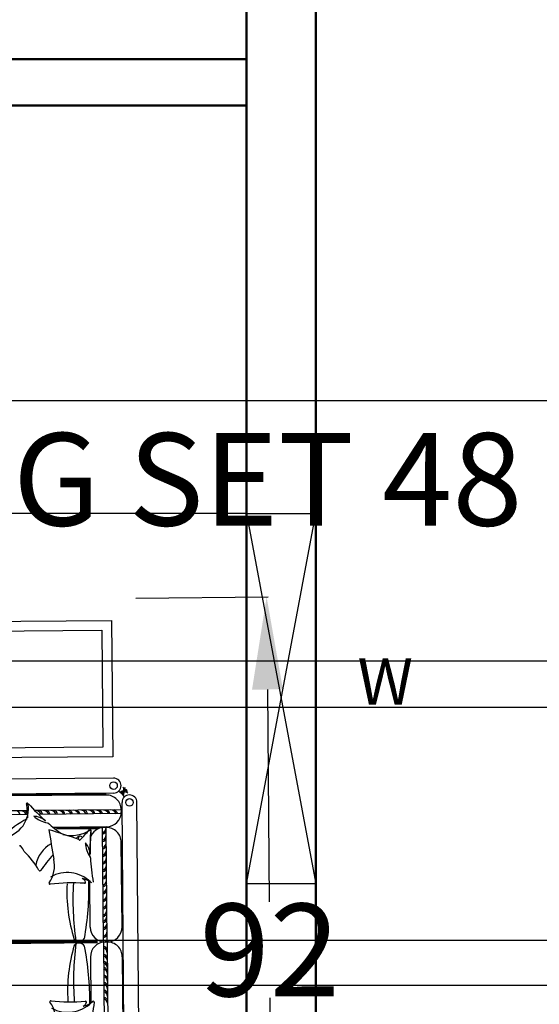
# Model space of a CAD drawing. Units: inches. Extents: x -77 to 516, y -119 to 536.
# Tile 9 of 11: x 335 to 403, y 159 to 287. Entities that reach past the tile are written whole.
import ezdxf

# ---------------------------------------------------------------- set-up
doc = ezdxf.new("R2010")
doc.units = ezdxf.units.IN
doc.header["$MEASUREMENT"] = 0
for name, color, linetype, lineweight in [('A-ANNO-DIMS', 2, 'Continuous', 18), ('furniture', 119, 'Continuous', 18), ('text', 170, 'Continuous', 18), ('walls', 40, 'Continuous', 50), ('windows', 1, 'Continuous', 25)]:
    doc.layers.add(name, color=color, linetype=linetype, lineweight=lineweight)
doc.layers.add('FUR', color=42, linetype='Continuous')
doc.styles.get("Standard").update_dxf_attribs({"font": 'arial.ttf'})
doc.dimstyles.get("Standard").update_dxf_attribs({"dimtxt": 12, "dimasz": 12, "dimexe": 0.18, "dimexo": 0.0625, "dimgap": 0.09, "dimtad": 0, "dimtih": 1, "dimtoh": 1, "dimdec": 1, "dimzin": 0, "dimdsep": 46, "dimlunit": 4, "dimtxsty": 'Standard', "dimcen": 0.09, "dimadec": 0, "dimazin": 0, "dimtfac": 1, "dimtdec": 1, "dimtofl": 0, "dimtmove": 0, "dimatfit": 3, "dimfxl": 1, "dimtolj": 1, "dimtzin": 0, "dimarcsym": 0})

# ---------------------------------------------------------------- blocks, each defined once
blk = doc.blocks.new('A$C44A37715')
at = {"layer": 'FUR'}
for p, q in [((0, 2.4786), (0, 1.048)), ((0.0768, 2.4786), (0.0768, 1.048)), ((0.1591, 1.763), (0.1591, 2.3508)), ((0.1783, 1.7636), (0.1783, 2.3502)), ((0.0822, 1.8399), (0.0822, 2.274)), ((0.2455, 1.8399), (0.2455, 2.0753)), ((0.1591, 1.764), (0.1687, 1.764)), ((0.1591, 1.764), (0.1687, 1.764)), ((0.1591, 1.7636), (0.1687, 1.7636)), ((0.1591, 1.7636), (0.1687, 1.7636)), ((0.1591, 1.7636), (0.1591, 1.1758)), ((0.1591, 1.763), (0.1687, 1.763)), ((0.1591, 1.7623), (0.1687, 1.7623)), ((0.1591, 1.7623), (0.1687, 1.7623)), ((0.1783, 1.763), (0.1783, 1.1764)), ((0.2091, 1.7681), (0.8452, 1.7681)), ((0.2091, 1.7681), (0.8452, 1.7681)), ((0.2091, 1.7633), (0.8487, 1.7633)), ((0.2091, 1.7585), (0.8452, 1.7585)), ((0.2103, 1.7681), (0.8452, 1.7681)), ((0.0822, 1.6868), (0.0822, 1.2527)), ((0.2455, 1.6868), (0.2455, 1.4514)), ((0.2446, 1.3239), (0.2446, 1.2958)), ((0.1577, 1.1727), (0.4308, 1.1727)), ((0.1591, 1.1758), (0.1687, 1.1758)), ((0.1845, 1.1775), (0.4249, 1.1775)), ((0.1995, 1.1823), (0.4138, 1.1823)), ((0.0809, 1.0862), (0.0809, 1.0958)), ((0.0809, 1.0862), (0.524, 1.0862)), ((0.0815, 1.1054), (0.5053, 1.1054)), ((0.5573, 1.0862), (0.8644, 1.0862)), ((0.56, 1.1054), (0.8638, 1.1054)), ((0.0809, 0.9614), (0.0809, 0.9614)), ((0.1193, 0.9998), (0.8259, 0.9998)), ((0.1577, 1.0094), (0.7875, 1.0094)), ((0.1577, 1.0046), (0.7875, 1.0046)), ((0.1193, 0.923), (0.8259, 0.923)), ((0.1193, 0.923), (0.8259, 0.923))]:
    blk.add_line(p, q, dxfattribs=at)
for points in [[(0.1226, 0.1134), (0.1226, 0.8134), (0.8226, 0.8134), (0.8226, 0.1134)], [(0.1726, 0.1634), (0.1726, 0.7634), (0.7726, 0.7634), (0.7726, 0.1634)]]:
    blk.add_lwpolyline(points, close=True, dxfattribs=at)
for centre in [(0.0384, 1.048), (0.1193, 0.9614)]:
    blk.add_circle(centre, 0.0192, dxfattribs=at)
for centre, radius, start, end in [((-0.7557, 2.2433), 0.9988, 350.147, 357.3879), ((0.5796, 2.1587), 0.1531, 167.3915, 215.6783), ((0.3624, 1.9521), 0.1703, 60.2042, 134.6584), ((0.1884, 2.0828), 0.0293, 181.8064, 249.8645), ((0.2331, 2.0716), 0.0048, 170.147, 311.7497), ((0.3028, 1.9936), 0.0998, 100.2155, 131.7497), ((1.732, 2.053), 1.4814, 179.0056, 190.4975), ((0.2725, 2.0713), 0.0048, 161.7015, 277.2637), ((0.2981, 2.0629), 0.0317, 114.2109, 161.7015), ((0.1823, 2.0725), 0.0245, 198.4382, 260.6098), ((0.1884, 2.0444), 0.0293, 181.8064, 249.8645), ((0.1823, 2.0341), 0.0245, 198.4382, 260.6098), ((0.3436, 1.1012), 0.9679, 83.706, 94.1744), ((-1.1315, 1.9749), 1.465, 351.9647, 3.6704), ((-0.4253, 2.0161), 0.7895, 342.552, 3.574), ((0.4506, 2.068), 0.0048, 259.041, 17.2752), ((0.1884, 2.006), 0.0293, 181.8064, 249.8645), ((0.1823, 1.9956), 0.0245, 198.4382, 260.6098), ((0.1884, 1.9676), 0.0293, 181.8064, 249.8645), ((0.1823, 1.9572), 0.0245, 198.4382, 260.6098), ((0.1884, 1.9292), 0.0293, 181.8064, 249.8645), ((0.1823, 1.9188), 0.0245, 198.4382, 260.6098), ((0.1884, 1.8972), 0.0293, 181.8064, 249.8645), ((0.1823, 1.8869), 0.0245, 198.4382, 260.6098), ((0.1591, 1.8399), 0.0768, 180, 270), ((0.1884, 1.8614), 0.0293, 181.8064, 249.8645), ((0.1823, 1.851), 0.0245, 198.4382, 260.6098), ((0.1884, 1.8204), 0.0293, 181.8064, 249.8645), ((0.1687, 1.8399), 0.0768, 270, 0), ((0.1823, 1.81), 0.0245, 198.4382, 260.6098), ((0.3031, 1.8009), 0.0329, 212.7236, 319.0819), ((0.1591, 1.6868), 0.0768, 90, 180), ((0.1823, 1.7166), 0.0245, 99.3902, 161.5618), ((0.1884, 1.7063), 0.0293, 110.1355, 178.1936), ((0.1687, 1.6868), 0.0768, 0, 90), ((1.7314, 1.4718), 1.4814, 169.3851, 180.877), ((0.3031, 1.7257), 0.0329, 40.9181, 147.2764), ((-1.1319, 1.5558), 1.465, 356.2122, 7.918), ((-0.4258, 1.5132), 0.7895, 356.3086, 17.3306), ((0.1823, 1.6756), 0.0245, 99.3902, 161.5618), ((0.1884, 1.6653), 0.0293, 110.1355, 178.1936), ((0.1823, 1.6398), 0.0245, 99.3902, 161.5618), ((0.1884, 1.6294), 0.0293, 110.1355, 178.1936), ((0.1823, 1.6078), 0.0245, 99.3902, 161.5618), ((0.1884, 1.5975), 0.0293, 110.1355, 178.1936), ((0.1823, 1.5694), 0.0245, 99.3902, 161.5618), ((0.1884, 1.5591), 0.0293, 110.1355, 178.1936), ((0.1823, 1.531), 0.0245, 99.3902, 161.5618), ((0.1884, 1.5207), 0.0293, 110.1355, 178.1936), ((0.1823, 1.4926), 0.0245, 99.3902, 161.5618), ((0.1884, 1.4822), 0.0293, 110.1355, 178.1936), ((0.1823, 1.4542), 0.0245, 99.3902, 161.5618), ((0.1884, 1.4438), 0.0293, 110.1355, 178.1936), ((0.1823, 1.4157), 0.0245, 99.3902, 161.5618), ((0.1884, 1.4054), 0.0293, 110.1355, 178.1936), ((-0.7567, 1.2866), 0.9988, 2.4947, 9.7356), ((0.3023, 1.5342), 0.0998, 228.1329, 259.6671), ((0.362, 1.5755), 0.1703, 225.2243, 299.6785), ((0.2719, 1.4565), 0.0048, 82.6189, 198.1812), ((0.2974, 1.4649), 0.0317, 198.1812, 245.6717), ((0.345, 2.4264), 0.9679, 265.7082, 276.1767), ((0.5787, 1.3685), 0.1531, 144.2044, 192.4911), ((0.45, 1.4595), 0.0048, 342.6074, 100.8416), ((0.1823, 1.3773), 0.0245, 99.3902, 161.5618), ((0.1884, 1.367), 0.0293, 110.1355, 178.1936), ((-0.251, 1.9276), 0.9195, 318.0608, 324.4706), ((0.3627, 1.399), 0.1625, 299.1576, 348.2707), ((0.5013, 1.3906), 0.0048, 28.9028, 147.137), ((0.8574, 1.5872), 0.4019, 208.9028, 226.4482), ((0.1823, 1.3389), 0.0245, 99.3902, 161.5618), ((0.1884, 1.3286), 0.0293, 110.1355, 178.1936), ((0.1823, 1.3005), 0.0245, 99.3902, 161.5618), ((0.1884, 1.2902), 0.0293, 110.1355, 178.1936), ((0.246, 1.3303), 0.0048, 182.4947, 215.9582), ((0.1413, 1.2543), 0.1246, 359.5452, 35.9582), ((-8.7106, -0.1777), 9.2643, 8.45789, 9.4001), ((0.1823, 1.2621), 0.0245, 99.3902, 161.5618), ((0.1884, 1.2517), 0.0293, 110.1355, 178.1936), ((-0.7567, 1.2866), 0.9988, 354.4679, 1.5003), ((-0.7557, 1.2833), 0.9988, 354.5852, 1.6176), ((0.3486, 1.3214), 0.1071, 184.6142, 219.4373), ((0.7534, 1.3788), 0.1918, 205.5948, 215.4865), ((0.6012, 1.2702), 0.0048, 215.4865, 326.8671), ((0.1591, 1.2527), 0.0768, 180, 270), ((0.1823, 1.2237), 0.0245, 99.3902, 161.5618), ((0.1884, 1.2133), 0.0293, 110.1355, 178.1936), ((0.1687, 1.2527), 0.0768, 270, 341.6974), ((0.338, 1.0263), 0.1892, 76.9024, 121.7844), ((0.9695, 0.5776), 0.9459, 135.7156, 139.9071), ((1.3243, 1.4687), 1.0743, 192.5844, 192.6033), ((0.2946, 1.2385), 0.0192, 222.5446, 329.0399), ((0.2958, 1.2347), 0.0048, 28.7142, 135.7156), ((-0.7444, 1.473), 1.0743, 346.3809, 347.1715), ((1.0961, 3.3234), 2.2331, 249.1159, 253.2608), ((0.7061, 1.0752), 0.1492, 97.8738, 190.1124), ((0.3864, 1.4953), 0.4082, 295.8111, 316.9977), ((0.1577, 1.0958), 0.0768, 90, 180), ((0.1823, 1.1852), 0.0245, 99.3902, 161.5618), ((0.1884, 1.1749), 0.0293, 110.1355, 178.1936), ((0.2423, 1.1899), 0.0048, 174.4679, 319.9071), ((0.2435, 1.1886), 0.0048, 174.5852, 320.0245), ((-0.2002, 0.3984), 0.9988, 48.7901, 53.8909), ((0.4435, 1.0253), 0.1246, 45.8406, 82.2536), ((-0.2002, 0.3984), 0.9988, 40.7632, 47.7957), ((0.5383, 1.2215), 0.1071, 230.9096, 265.7327), ((1.505, 1.1564), 0.9459, 182.0299, 186.0564), ((0.1577, 1.0862), 0.0768, 180, 270), ((0.125, 1.1094), 0.0245, 189.3902, 251.5618), ((0.1354, 1.1155), 0.0293, 200.1355, 268.1936), ((0.1635, 1.1094), 0.0245, 189.3902, 251.5618), ((0.1738, 1.1155), 0.0293, 200.1355, 268.1936), ((0.2019, 1.1094), 0.0245, 189.3902, 251.5618), ((0.2122, 1.1155), 0.0293, 200.1355, 268.1936), ((0.2403, 1.1094), 0.0245, 189.3902, 251.5618), ((0.2506, 1.1155), 0.0293, 200.1355, 268.1936), ((0.2787, 1.1094), 0.0245, 189.3902, 251.5618), ((0.289, 1.1155), 0.0293, 200.1355, 268.1936), ((0.3171, 1.1094), 0.0245, 189.3902, 251.5618), ((0.3275, 1.1155), 0.0293, 200.1355, 268.1936), ((0.3555, 1.1094), 0.0245, 189.3902, 251.5618), ((0.3659, 1.1155), 0.0293, 200.1355, 268.1936), ((0.394, 1.1094), 0.0245, 189.3902, 251.5618), ((0.4043, 1.1155), 0.0293, 200.1355, 268.1936), ((0.4324, 1.1094), 0.0245, 189.3902, 251.5618), ((0.4427, 1.1155), 0.0293, 200.1355, 268.1936), ((0.4708, 1.1094), 0.0245, 189.3902, 251.5618), ((0.4811, 1.1155), 0.0293, 200.1355, 268.1936), ((0.5092, 1.1094), 0.0245, 189.3902, 251.5618), ((0.5195, 1.1155), 0.0293, 200.1355, 268.1936), ((0.586, 1.1094), 0.0245, 189.3902, 251.5618), ((0.5964, 1.1155), 0.0293, 200.1355, 268.1936), ((0.6245, 1.1094), 0.0245, 189.3902, 251.5618), ((0.0384, 1.048), 0.0384, 180, 270), ((0.0384, 1.048), 0.0384, 270, 0), ((0.1577, 1.0862), 0.1152, 215.5109, 236.4018), ((0.5628, 1.0521), 0.0048, 220.7632, 70.652), ((0.0673, 1.0212), 0.0288, 223.4628, 270.6626), ((0.0466, 0.9924), 0.00508, 306.6856, 50.7244), ((0.0585, 0.9912), 0.00925, 197.7913, 7.4173), ((0.0606, 0.9941), 0.00723, 150.0455, 345.9236), ((0.0576, 0.9851), 0.0124, 280.1683, 35.9879), ((0.0778, 0.9831), 0.0137, 137.5189, 242.0632), ((0.0743, 0.9993), 0.0096, 101.3851, 350.9956), ((0.075, 0.9999), 0.0048, 71.6913, 20.8298), ((0.1193, 0.9614), 0.0384, 90, 180), ((0.1193, 0.9614), 0.0384, 180, 270)]:
    blk.add_arc(centre, radius, start, end, dxfattribs=at)
blk = doc.blocks.new('WIN-48IN')
for p, q in [((0, 0), (9, 48)), ((0, 48), (9, 0))]:
    blk.add_line(p, q)
blk.add_lwpolyline([(0, 48), (9, 48), (9, 0), (0, 0)], close=True)
blk = doc.blocks.new('*D31')
at = {"layer": 'A-ANNO-DIMS', "color": 0, "lineweight": -2, "transparency": 16777216}
for p, q in [((350.4, 211.74), (367.54, 211.89)), ((367.47, 199.89), (367.71, 172.35)), ((368.05, 132.38), (367.82, 159.91)), ((351.2, 120.23), (368.34, 120.38))]:
    blk.add_line(p, q, dxfattribs=at)
at = {"layer": 'A-ANNO-DIMS', "color": 0, "transparency": 16777216}
for points in [[(369.47, 199.9), (365.47, 199.87), (367.36, 211.88)], [(370.05, 132.4), (366.05, 132.36), (368.16, 120.38)]]:
    blk.add_solid(points, dxfattribs=at)
at = {"layer": 'Defpoints', "color": 0, "transparency": 16777216}
for p in [(350.34, 211.74), (351.13, 120.23), (368.16, 120.38)]:
    blk.add_point(p, dxfattribs=at)
at = {"layer": 'A-ANNO-DIMS', "color": 0, "transparency": 16777216, "insert": (367.76, 166.13), "char_height": 12, "attachment_point": 5}
blk.add_mtext('\\A1;92', dxfattribs=at)
blk = doc.blocks.new('*D32')
at = {"layer": 'A-ANNO-DIMS', "color": 0, "lineweight": -2, "transparency": 16777216}
for p, q in [((226.61, 234.25), (226.61, 226.94)), ((274.55, 234.25), (274.55, 226.94)), ((238.61, 227.12), (262.55, 227.12)), ((274.55, 227.12), (286.55, 227.12))]:
    blk.add_line(p, q, dxfattribs=at)
at = {"layer": 'A-ANNO-DIMS', "color": 0, "transparency": 16777216}
for points in [[(238.61, 229.12), (238.61, 225.12), (226.61, 227.12)], [(262.55, 229.12), (262.55, 225.12), (274.55, 227.12)]]:
    blk.add_solid(points, dxfattribs=at)
at = {"layer": 'Defpoints', "color": 0, "transparency": 16777216}
for p in [(226.61, 234.31), (274.55, 234.31), (274.55, 227.12)]:
    blk.add_point(p, dxfattribs=at)
at = {"layer": 'A-ANNO-DIMS', "color": 0, "transparency": 16777216, "insert": (345.24, 227.12), "char_height": 12, "attachment_point": 5}
blk.add_mtext('\\A1;DINING SET 48', dxfattribs=at)
blk = doc.blocks.new('*D37')
at = {"layer": 'A-ANNO-DIMS', "color": 0, "lineweight": -2, "transparency": 16777216}
for p, q in [((373.81, 494.59), (454.58, 494.59)), ((454.4, 482.59), (454.4, 212.81)), ((454.4, -69.41), (454.4, 200.37)), ((309, -81.41), (454.58, -81.41))]:
    blk.add_line(p, q, dxfattribs=at)
at = {"layer": 'A-ANNO-DIMS', "color": 0, "transparency": 16777216}
for points in [[(452.4, 482.59), (456.4, 482.59), (454.4, 494.59)], [(452.4, -69.41), (456.4, -69.41), (454.4, -81.41)]]:
    blk.add_solid(points, dxfattribs=at)
at = {"layer": 'Defpoints', "color": 0, "transparency": 16777216}
for p in [(373.75, 494.59), (454.4, 494.59), (308.93, -81.41)]:
    blk.add_point(p, dxfattribs=at)
at = {"layer": 'A-ANNO-DIMS', "color": 0, "transparency": 16777216, "insert": (454.4, 206.59), "char_height": 12, "attachment_point": 5}
blk.add_mtext('\\A1;576', dxfattribs=at)
blk = doc.blocks.new('*D42')
at = {"layer": 'A-ANNO-DIMS', "color": 0, "lineweight": -2, "transparency": 16777216}
for p, q in [((454.4, 197.59), (454.4, 209.59)), ((454.4, 209.59), (466.4, 209.59)), ((22.81, 197.59), (454.58, 197.59)), ((454.4, 179.41), (454.4, 185.59)), ((22.81, 167.41), (454.58, 167.41))]:
    blk.add_line(p, q, dxfattribs=at)
at = {"layer": 'A-ANNO-DIMS', "color": 0, "transparency": 16777216}
for points in [[(452.4, 185.59), (456.4, 185.59), (454.4, 197.59)], [(452.4, 179.41), (456.4, 179.41), (454.4, 167.41)]]:
    blk.add_solid(points, dxfattribs=at)
at = {"layer": 'Defpoints', "color": 0, "transparency": 16777216}
for p in [(22.75, 197.59), (454.4, 197.59), (22.75, 167.41)]:
    blk.add_point(p, dxfattribs=at)
at = {"layer": 'A-ANNO-DIMS', "color": 0, "transparency": 16777216, "insert": (486.75, 209.59), "char_height": 12, "attachment_point": 5}
blk.add_mtext('\\A1;30.18', dxfattribs=at)
blk = doc.blocks.new('*D43')
at = {"layer": 'A-ANNO-DIMS', "color": 0, "lineweight": -2, "transparency": 16777216}
for p, q in [((454.4, 237.36), (454.4, 249.36)), ((454.4, 249.36), (466.4, 249.36)), ((22.81, 237.36), (454.58, 237.36)), ((454.4, 215.59), (454.4, 225.36)), ((22.81, 203.59), (454.58, 203.59))]:
    blk.add_line(p, q, dxfattribs=at)
at = {"layer": 'A-ANNO-DIMS', "color": 0, "transparency": 16777216}
for points in [[(452.4, 225.36), (456.4, 225.36), (454.4, 237.36)], [(452.4, 215.59), (456.4, 215.59), (454.4, 203.59)]]:
    blk.add_solid(points, dxfattribs=at)
at = {"layer": 'Defpoints', "color": 0, "transparency": 16777216}
for p in [(22.75, 237.36), (454.4, 237.36), (22.75, 203.59)]:
    blk.add_point(p, dxfattribs=at)
at = {"layer": 'A-ANNO-DIMS', "color": 0, "transparency": 16777216, "insert": (491.44, 249.36), "char_height": 12, "attachment_point": 5}
blk.add_mtext('\\A1;33.775', dxfattribs=at)
blk = doc.blocks.new('*D47')
at = {"layer": 'A-ANNO-DIMS', "color": 0, "lineweight": -2, "transparency": 16777216}
for p, q in [((364.69, 275.59), (-16.08, 275.59)), ((-15.9, 263.59), (-15.9, 255.37)), ((-15.9, 234.71), (-15.9, 242.93)), ((364.69, 222.71), (-16.08, 222.71))]:
    blk.add_line(p, q, dxfattribs=at)
at = {"layer": 'A-ANNO-DIMS', "color": 0, "transparency": 16777216}
for points in [[(-17.9, 263.59), (-13.9, 263.59), (-15.9, 275.59)], [(-17.9, 234.71), (-13.9, 234.71), (-15.9, 222.71)]]:
    blk.add_solid(points, dxfattribs=at)
at = {"layer": 'Defpoints', "color": 0, "transparency": 16777216}
for p in [(-15.9, 275.59), (364.75, 275.59), (364.75, 222.71)]:
    blk.add_point(p, dxfattribs=at)
at = {"layer": 'A-ANNO-DIMS', "color": 0, "transparency": 16777216, "insert": (-15.9, 249.15), "char_height": 12, "attachment_point": 5}
blk.add_mtext('\\A1;52.87', dxfattribs=at)
blk = doc.blocks.new('*D48')
at = {"layer": 'A-ANNO-DIMS', "color": 0, "lineweight": -2, "transparency": 16777216}
for p, q in [((364.69, 323.24), (-16.08, 323.24)), ((-15.9, 311.24), (-15.9, 308.63)), ((-15.9, 293.59), (-15.9, 296.2)), ((364.69, 281.59), (-16.08, 281.59))]:
    blk.add_line(p, q, dxfattribs=at)
at = {"layer": 'A-ANNO-DIMS', "color": 0, "transparency": 16777216}
for points in [[(-17.9, 311.24), (-13.9, 311.24), (-15.9, 323.24)], [(-17.9, 293.59), (-13.9, 293.59), (-15.9, 281.59)]]:
    blk.add_solid(points, dxfattribs=at)
at = {"layer": 'Defpoints', "color": 0, "transparency": 16777216}
for p in [(-15.9, 323.24), (364.75, 323.24), (364.75, 281.59)]:
    blk.add_point(p, dxfattribs=at)
at = {"layer": 'A-ANNO-DIMS', "color": 0, "transparency": 16777216, "insert": (-15.9, 302.42), "char_height": 12, "attachment_point": 5}
blk.add_mtext('\\A1;41.65', dxfattribs=at)
blk = doc.blocks.new('*D55')
at = {"layer": 'A-ANNO-DIMS', "color": 0, "lineweight": -2, "transparency": 16777216}
for p, q in [((454.4, 197.59), (454.4, 209.59)), ((454.4, 209.59), (466.4, 209.59)), ((163.81, 197.59), (454.58, 197.59)), ((454.4, 173.59), (454.4, 185.59)), ((163.81, 161.59), (454.58, 161.59))]:
    blk.add_line(p, q, dxfattribs=at)
at = {"layer": 'A-ANNO-DIMS', "color": 0, "transparency": 16777216}
for points in [[(452.4, 185.59), (456.4, 185.59), (454.4, 197.59)], [(452.4, 173.59), (456.4, 173.59), (454.4, 161.59)]]:
    blk.add_solid(points, dxfattribs=at)
at = {"layer": 'Defpoints', "color": 0, "transparency": 16777216}
for p in [(163.75, 197.59), (454.4, 197.59), (163.75, 161.59)]:
    blk.add_point(p, dxfattribs=at)
at = {"layer": 'A-ANNO-DIMS', "color": 0, "transparency": 16777216, "insert": (475.08, 209.59), "char_height": 12, "attachment_point": 5}
blk.add_mtext('\\A1;36', dxfattribs=at)
blk = doc.blocks.new('*D56')
at = {"layer": 'A-ANNO-DIMS', "color": 0, "lineweight": -2, "transparency": 16777216}
for p, q in [((454.4, 215.59), (454.4, 227.59)), ((454.4, 227.59), (466.4, 227.59)), ((157.81, 203.59), (454.58, 203.59)), ((157.81, 197.59), (454.58, 197.59)), ((454.4, 185.59), (454.4, 173.59))]:
    blk.add_line(p, q, dxfattribs=at)
at = {"layer": 'A-ANNO-DIMS', "color": 0, "transparency": 16777216}
for points in [[(452.4, 215.59), (456.4, 215.59), (454.4, 203.59)], [(452.4, 185.59), (456.4, 185.59), (454.4, 197.59)]]:
    blk.add_solid(points, dxfattribs=at)
at = {"layer": 'Defpoints', "color": 0, "transparency": 16777216}
for p in [(157.75, 203.59), (454.4, 203.59), (157.75, 197.59)]:
    blk.add_point(p, dxfattribs=at)
at = {"layer": 'A-ANNO-DIMS', "color": 0, "transparency": 16777216, "insert": (470.45, 227.59), "char_height": 12, "attachment_point": 5}
blk.add_mtext('\\A1;6', dxfattribs=at)

msp = doc.modelspace()

# ---------------------------------------------------------------- linework, layer by layer
at = {"layer": 'walls'}
for p, q in [((364.7501, 131.5884), (364.7501, 485.5884)), ((364.7501, 281.5884), (229.7501, 281.5884)), ((364.7501, 275.5884), (223.7501, 275.5884))]:
    msp.add_line(p, q, dxfattribs=at)
msp.add_lwpolyline([(373.7501, 131.5884), (373.7501, 494.5884), (13.7501, 494.5884), (13.7501, 14.5884), (239.7501, 14.5884)], dxfattribs=at)

# ---------------------------------------------------------------- block references
at = {"layer": 'furniture', "xscale": 25.25763254760833, "yscale": 25.25763254760833, "zscale": 25.25763254760833, "rotation": 180.4978074292498}
msp.add_blockref('A$C44A37715', (350.3392, 211.7368), dxfattribs=at)
at = {"layer": 'windows'}
msp.add_blockref('WIN-48IN', (364.75, 174.7142), dxfattribs=at)

# ---------------------------------------------------------------- texts
at = {"layer": 'text', "insert": (379.1328, 203.9098), "char_height": 6, "attachment_point": 1}
msp.add_mtext_dynamic_manual_height_columns('W', width=105.041962, gutter_width=1, heights=[0], dxfattribs=at)

# ---------------------------------------------------------------- dimensions: what is measured, and where the dimension line sits
at = {"layer": 'A-ANNO-DIMS'}
for base, p1, p2, angle, override, picture, middle in [((454.4001, 494.5884), (308.9336, -81.4116), (373.7501, 494.5884), 90, {"dimdec": 0, "dimlfac": 1, "dimrnd": 0, "dimzin": 0, "dimdsep": 46, "dimlunit": 2}, '*D37', (454.4001, 206.5884)), ((-15.8999, 323.2426), (364.7501, 281.5884), (364.7501, 323.2426), 90, {"dimdec": 2, "dimlfac": 1, "dimrnd": 0, "dimzin": 0, "dimdsep": 46, "dimlunit": 2}, '*D48', (-15.8999, 302.4155)), ((-15.8999, 275.5884), (364.7501, 222.7137), (364.7501, 275.5884), 90, {"dimdec": 2, "dimlfac": 1, "dimrnd": 0, "dimzin": 0, "dimdsep": 46, "dimlunit": 2}, '*D47', (-15.8999, 249.151)), ((454.4001, 237.3631), (22.7501, 203.5884), (22.7501, 237.3631), 90, {"dimdec": 3, "dimlfac": 1, "dimrnd": 0, "dimzin": 0, "dimdsep": 46, "dimlunit": 2}, '*D43', (491.4396, 249.3631)), ((454.4001, 203.5884), (157.7501, 197.5884), (157.7501, 203.5884), 90, {"dimdec": 0, "dimlfac": 1, "dimrnd": 0, "dimzin": 0, "dimdsep": 46, "dimlunit": 2}, '*D56', (470.4519, 227.5884)), ((454.4001, 197.5884), (22.7501, 167.4079), (22.7501, 197.5884), 90, {"dimdec": 2, "dimlfac": 1, "dimrnd": 0, "dimzin": 0, "dimdsep": 46, "dimlunit": 2}, '*D42', (486.7452, 209.5884)), ((454.4001, 197.5884), (163.7501, 161.5884), (163.7501, 197.5884), 90, {"dimdec": 0, "dimlfac": 1, "dimrnd": 0, "dimzin": 0, "dimdsep": 46, "dimlunit": 2}, '*D55', (475.0767, 209.5884)), ((368.159, 120.3789), (350.3392, 211.7368), (351.1342, 120.231), 270.497807, {"dimdec": 0, "dimlfac": 1, "dimrnd": 0, "dimzin": 0, "dimdsep": 46, "dimlunit": 2}, '*D31', (367.7615, 166.1318))]:
    dim = msp.add_linear_dim(base=base, p1=p1, p2=p2, angle=angle, dimstyle='Standard', override=override, dxfattribs=at)
    dim.commit()
    dim.dimension.update_dxf_attribs({"geometry": picture, "text_midpoint": middle})
dim = msp.add_linear_dim(base=(274.5499, 227.1182), p1=(226.6056, 234.3099), p2=(274.5499, 234.3099), text='DINING SET <>', dimstyle='Standard', override={"dimdec": 0, "dimlfac": 1, "dimrnd": 0, "dimzin": 0, "dimdsep": 46, "dimlunit": 2}, dxfattribs=at)
dim.commit()
dim.dimension.update_dxf_attribs({"geometry": '*D32', "text_midpoint": (345.2442, 227.1182)})

doc.saveas('drawing.dxf')
